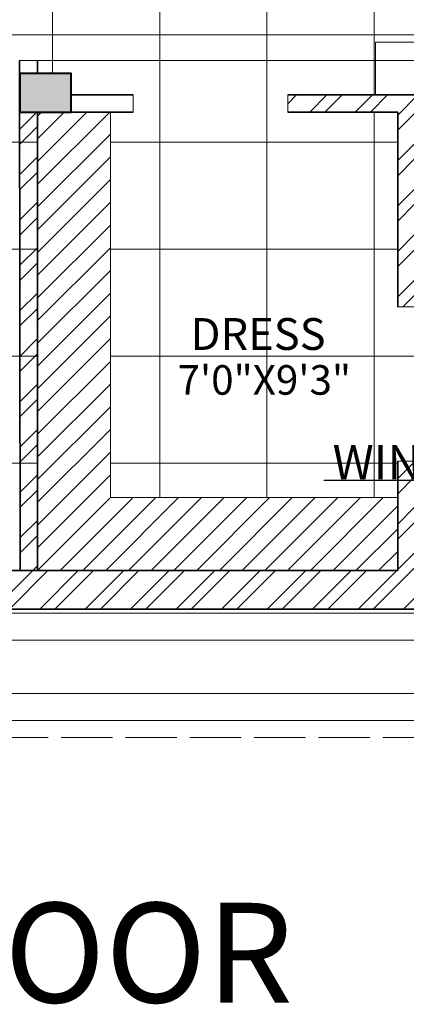
# Model space of a CAD drawing. Units: inches. Extents: x 351 to 1738, y -265 to 286.
# Tile 29 of 38: x 1380 to 1470, y -265 to -35. Entities that reach past the tile are written whole.
import ezdxf

# ---------------------------------------------------------------- set-up
doc = ezdxf.new("R2010")
doc.units = ezdxf.units.IN
doc.header["$MEASUREMENT"] = 0
doc.linetypes.add('ACAD_ISO02W100', pattern=[15, 12, -3])
for name, color, linetype, lineweight in [('A-ANNO-DIMS', 2, 'Continuous', 18), ('A-ANNO-TITL', 7, 'Continuous', 35), ('A-AREA-IDEN', 7, 'Continuous', 18), ('A-COLS', 7, 'Continuous', 40), ('A-COLS-PATT', 6, 'Continuous', 13), ('A-DOOR', 3, 'Continuous', 18), ('A-FLOR-CASE', 9, 'Continuous', 18), ('A-FLOR-CASE-PATT', 9, 'Continuous', 9), ('A-FLOR-OVHD', 1, 'ACAD_ISO02W100', 18), ('A-FLOR-PATT', 9, 'Continuous', 9), ('A-WALL', 7, 'Continuous', 35), ('A-WALL-PATT', 152, 'Continuous', 13)]:
    doc.layers.add(name, color=color, linetype=linetype, lineweight=lineweight)
doc.styles.add('Annotative', font='arial.ttf')
doc.styles.get("Standard").update_dxf_attribs({"font": 'arial.ttf'})
doc.dimstyles.get("Standard").update_dxf_attribs({"dimtxt": 8, "dimasz": 5, "dimexe": 0.18, "dimexo": 0.0625, "dimgap": 0.09, "dimtad": 1, "dimtoh": 1, "dimzin": 0, "dimdsep": 46, "dimlunit": 4, "dimtxsty": 'Standard', "dimcen": 0, "dimclre": 256, "dimadec": 0, "dimazin": 0, "dimtfac": 1, "dimtofl": 0, "dimtmove": 0, "dimatfit": 3, "dimfxl": 1, "dimtolj": 1, "dimtzin": 0, "dimlwe": -1, "dimarcsym": 0})

# ---------------------------------------------------------------- blocks, each defined once
blk = doc.blocks.new('CONSOLE-TV')
blk.add_lwpolyline([(0, 0), (61, 0), (61, 12.29), (0, 12.29)], close=True)
blk = doc.blocks.new('COL-9x12')
blk.add_lwpolyline([(0, 12), (0, 0), (9, 0), (9, 12)], close=True)
blk = doc.blocks.new('*D32')
at = {"layer": 'A-ANNO-DIMS', "transparency": 16777216}
for p, q in [((1557.64, -102), (1552.12, -102)), ((1557.64, -138), (1552.12, -138))]:
    blk.add_line(p, q, dxfattribs=at)
at = {"layer": 'A-ANNO-DIMS', "color": 0, "lineweight": -2, "transparency": 16777216}
for p, q in [((1552.3, -107), (1552.3, -133)), ((1552.3, -138), (1552.3, -143)), ((1552.3, -143), (1450.98, -143))]:
    blk.add_line(p, q, dxfattribs=at)
at = {"layer": 'A-ANNO-DIMS', "color": 0, "transparency": 16777216}
for points in [[(1551.47, -107), (1553.14, -107), (1552.3, -102)], [(1551.47, -133), (1553.14, -133), (1552.3, -138)]]:
    blk.add_solid(points, dxfattribs=at)
at = {"layer": 'Defpoints', "color": 0, "transparency": 16777216}
for p in [(1557.7, -102), (1552.3, -138), (1557.7, -138)]:
    blk.add_point(p, dxfattribs=at)
at = {"layer": 'A-ANNO-DIMS', "color": 0, "transparency": 16777216, "insert": (1501.6, -138.77), "char_height": 8, "attachment_point": 5}
blk.add_mtext('\\A1;WINDOW 3\'-0" TYP.', dxfattribs=at)
blk = doc.blocks.new('*D66')
at = {"layer": 'A-ANNO-DIMS', "transparency": 16777216}
for p, q in [((1384.27, -3.5), (1596.33, -3.5)), ((1384.27, -45), (1596.33, -45))]:
    blk.add_line(p, q, dxfattribs=at)
at = {"layer": 'A-ANNO-DIMS', "color": 0, "lineweight": -2, "transparency": 16777216}
blk.add_line((1596.15, -40), (1596.15, -8.5), dxfattribs=at)
at = {"layer": 'A-ANNO-DIMS', "color": 0, "transparency": 16777216}
for points in [[(1595.32, -8.5), (1596.99, -8.5), (1596.15, -3.5)], [(1595.32, -40), (1596.99, -40), (1596.15, -45)]]:
    blk.add_solid(points, dxfattribs=at)
at = {"layer": 'Defpoints', "color": 0, "transparency": 16777216}
for p in [(1384.2, -3.5), (1596.15, -3.5), (1384.2, -45)]:
    blk.add_point(p, dxfattribs=at)
at = {"layer": 'A-ANNO-DIMS', "color": 0, "transparency": 16777216, "insert": (1591.92, -24.25), "char_height": 8, "attachment_point": 5, "rotation": 90}
blk.add_mtext('\\A1;3\'-5 1/2"', dxfattribs=at)

msp = doc.modelspace()

# ---------------------------------------------------------------- hatches: boundary and pattern name
at = {"layer": 'A-COLS-PATT'}
h = msp.add_hatch(color=256, dxfattribs=at)
h.dxf.hatch_style = 1
h.paths.add_polyline_path([(1112.704, 237.963), (1103.704, 237.963), (1103.704, 228.963), (1112.704, 228.963)])
h.paths.add_polyline_path([(1115.704, 237.963), (1112.704, 237.963), (1112.704, 228.963), (1115.704, 228.963)])
h.paths.add_polyline_path([(1043.704, 255.963), (1034.704, 255.963), (1034.704, 243.963), (1043.704, 243.963)])
h.paths.add_polyline_path([(1043.704, 210.963), (1034.704, 210.963), (1034.704, 198.963), (1043.704, 198.963)])
h.paths.add_polyline_path([(1043.704, -45.037), (1034.704, -45.037), (1034.704, -57.037), (1043.704, -57.037)])
h.paths.add_polyline_path([(1112.704, -45.037), (1103.704, -45.037), (1103.704, -57.037), (1112.704, -57.037)])
h.paths.add_polyline_path([(1112.704, -161.037), (1103.704, -161.037), (1103.704, -164.037), (1103.704, -173.037), (1112.704, -173.037)])
h.paths.add_polyline_path([(1043.704, -161.037), (1034.704, -161.037), (1034.704, -173.037), (1043.704, -173.037)])
h.paths.add_polyline_path([(1248.549, -164.037), (1236.549, -164.037), (1236.549, -173.037), (1248.549, -173.037)])
h.paths.add_polyline_path([(1248.549, -50), (1236.549, -50), (1236.549, -59), (1248.549, -59)])
h.paths.add_polyline_path([(1248.704, 73.463), (1244.704, 73.463), (1244.704, 64.463), (1248.704, 64.463)])
h.paths.add_polyline_path([(1244.704, 73.463), (1236.704, 73.463), (1236.704, 64.463), (1244.704, 64.463)])
h.paths.add_polyline_path([(1248.704, 237.963), (1236.704, 237.963), (1236.704, 228.963), (1248.704, 228.963)])
h.paths.add_polyline_path([(1392.204, 237.963), (1380.204, 237.963), (1380.204, 228.963), (1392.204, 228.963)])
h.paths.add_polyline_path([(1536.064, 237.963), (1524.064, 237.963), (1524.064, 228.963), (1536.064, 228.963)])
h.paths.add_polyline_path([(1536.064, 73.463), (1524.064, 73.463), (1524.064, 64.463), (1536.064, 64.463)])
h.paths.add_polyline_path([(1384.204, 73.463), (1380.204, 73.463), (1380.204, 64.463), (1384.204, 64.463)])
h.paths.add_polyline_path([(1392.064, 73.463), (1384.204, 73.463), (1384.204, 64.463), (1392.064, 64.463)])
h.paths.add_polyline_path([(1536.064, -53.037), (1524.064, -53.037), (1524.064, -57.037), (1536.064, -57.037)])
h.paths.add_polyline_path([(1536.064, -48.037), (1524.064, -48.037), (1524.064, -53.037), (1536.064, -53.037)])
h.paths.add_polyline_path([(1392.064, -48.037), (1380.064, -48.037), (1380.064, -56.5), (1380.065, -57.037), (1392.064, -57.037)])
h.paths.add_polyline_path([(1536.064, -164.037), (1524.064, -164.037), (1524.064, -173.037), (1536.064, -173.037)])
at = {"layer": 'A-FLOR-CASE-PATT'}
h = msp.add_hatch(dxfattribs=at)
h.set_pattern_fill('ANSI31', color=256, scale=30)
h.set_pattern_definition([(45, (1384.204, -164.0373), (-2.65165, 2.65165), [])])
h.paths.add_polyline_path([(1401.204, -57.037), (1384.204, -57.037), (1384.204, -164.037), (1468.204, -164.037), (1468.204, -147.037), (1401.204, -147.037)])
at = {"layer": 'A-FLOR-PATT', "transparency": 33554559}
h = msp.add_hatch(dxfattribs=at)
h.set_pattern_fill('ANSI37', color=256, scale=200, angle=135)
h.set_pattern_definition([(180, (1112.704, -164.037), (-2e-15, -25), []), (270, (1112.704, -164.037), (25, -5e-15), [])])
h.paths.add_polyline_path([(1380.064, 73.463), (1380.132, 148.463), (1338.064, 148.463), (1290.704, 148.463), (1290.704, 88.463), (1248.704, 88.463), (1248.704, -2.009), (1244.704, -2.009), (1244.704, 142.457), (1160.704, 142.457), (1160.704, 158.963), (1160.704, 170.137), (1160.704, 206.137), (1160.704, 228.963), (1112.704, 228.963), (1112.704, 209.963), (1112.704, 168.963), (1124.704, 168.963), (1124.704, 162.963), (1112.704, 162.963), (1112.704, 64.463), (1112.704, 60.463), (1112.704, 0.463), (1112.704, -48.026), (1146.804, -47.981), (1146.804, -35.691), (1207.804, -35.691), (1207.804, -47.902), (1236.542, -47.864), (1236.544, -50.009), (1248.5, -50.009), (1248.506, -102.915), (1248.512, -150.915), (1248.514, -164.037), (1248.549, -164.037), (1273.017, -164.037), (1273.017, -128.799), (1355.24, -128.799), (1355.24, -164.037), (1384.204, -164.037), (1384.204, -57.037), (1380.064, -57.037), (1380.064, -48.037), (1392.064, -48.037), (1392.064, -53.037), (1406.549, -53.037), (1406.549, -57.037), (1401.204, -57.037), (1401.204, -147.037), (1468.204, -147.037), (1468.204, -138.5), (1472.204, -138.5), (1472.204, -102.5), (1468.204, -102.5), (1468.204, -57.037), (1442.549, -57.037), (1442.549, -53.037), (1463.049, -53.037), (1463.049, -40.747), (1524.049, -40.747), (1524.049, -48.037), (1536.064, -48.037), (1536.064, -53.037), (1557.704, -53.037), (1557.704, 204.963), (1384.204, 204.963), (1384.204, 73.463), (1392.064, 73.463), (1392.064, 64.463), (1384.204, 64.463), (1384.204, -3.5), (1380.204, -3.537), (1380.204, 64.463), (1380.064, 64.463)])
h.paths.add_polyline_path([(1510.714, 86.458, -0.1039845), (1511.661, 85.595, 0.4704384), (1510.158, 87.614, 0.0961001)], flags=16)
h.paths.add_polyline_path([(1510.443, 100.266, 0.009798), (1504.693, 100.48, 0.0287898), (1504.6, 99.767, -0.1653311), (1505.519, 96.135, -0.1436014)], flags=16)
h.paths.add_polyline_path([(1487.201, 85.595, -0.1039845), (1488.148, 86.458, 0.0961001), (1488.704, 87.614, 0.4704384)], flags=0)
h.paths.add_polyline_path([(1495.052, 100.43), (1494.178, 100.43, -0.0264629), (1494.262, 99.774, -0.1442193)], flags=16)
h.paths.add_polyline_path([(1444.485, 86.458, -0.1039845), (1445.433, 85.595, 0.4704384), (1443.93, 87.614, 0.0961001)], flags=16)
h.paths.add_polyline_path([(1420.972, 85.595, -0.1039845), (1421.92, 86.458, 0.0961001), (1422.475, 87.614, 0.4704384)], flags=16)
h.paths.add_polyline_path([(1428.632, 100.335, 0.0010541), (1427.971, 100.309, -0.0215241), (1428.033, 99.774, -0.1143008)], flags=16)
h.paths.add_polyline_path([(1419.906, 143.708, 0.0249793), (1420.222, 157.526), (1421.573, 159.101), (1421.573, 175.369), (1391.393, 175.369), (1391.393, 200.519), (1542.294, 200.519), (1542.294, 175.369), (1512.028, 175.369, 0.0198653), (1511.521, 153.838, 0.0251335), (1512.758, 118.323, 0.0205529), (1512.942, 115.253), (1419.834, 115.253, -0.0004142), (1419.843, 124.798), (1413.059, 124.798), (1413.059, 84.437, -0.0618528), (1415.831, 80.45, -0.0930773), (1420.972, 85.595, -0.2675367), (1422.371, 84.732, 0.0851103), (1424.052, 84.616, -0.8853927), (1424.033, 84.851, -1.1258145), (1424.073, 84.366, -0.0879871), (1422.371, 84.732, -0.2675367), (1422.326, 83.089, -0.3705421), (1420.972, 85.595, 0.0930773), (1415.831, 80.45, -0.0874142), (1417.914, 73.937), (1418.941, 73.937, 0.0272504), (1418.913, 76.906, -0.1157032), (1421.051, 73.937), (1445.354, 73.937, -0.1157032), (1447.492, 76.906, 0.0272504), (1447.464, 73.937), (1448.491, 73.937, -0.0874142), (1450.574, 80.45, 0.0930773), (1445.433, 85.595, -0.3705421), (1444.079, 83.089, -0.2675367), (1444.034, 84.732, -0.0879871), (1442.332, 84.366, -1.1258145), (1442.372, 84.851, -2.0327363), (1442.364, 84.368, 0.0863779), (1444.034, 84.732, -0.2675367), (1445.433, 85.595, -0.0930773), (1450.574, 80.45, -0.2577317), (1466.483, 90.927, -0.4786702), (1468.832, 91.907, -0.4786702), (1471.18, 90.927, -0.26264), (1483.053, 81.78, -0.0718662), (1487.201, 85.595, -0.2675367), (1488.6, 84.732, 0.0851103), (1490.28, 84.616, -0.8853927), (1490.262, 84.851, -1.1258145), (1490.301, 84.366, -0.0879871), (1488.6, 84.732, -0.2675367), (1488.554, 83.089, -0.3705421), (1487.201, 85.595, 0.0718662), (1483.053, 81.78, -0.1320648), (1484.143, 73.937), (1485.169, 73.937, 0.0272504), (1485.142, 76.906, -0.1157032), (1487.28, 73.937), (1511.582, 73.937, -0.1157032), (1513.72, 76.906, 0.0272504), (1513.693, 73.937), (1514.719, 73.937, -0.0874142), (1516.802, 80.45, 0.0930773), (1511.661, 85.595, -0.3705421), (1510.308, 83.089, -0.2675367), (1510.262, 84.732, -0.0879871), (1508.561, 84.366, -1.1258145), (1508.601, 84.851, -2.0327363), (1508.592, 84.368, 0.0863779), (1510.262, 84.732, -0.2675367), (1511.661, 85.595, -0.0930773), (1516.802, 80.45, -0.0618528), (1519.575, 84.437), (1519.575, 73.937), (1413.059, 73.937), (1413.059, 124.798), (1419.843, 124.798, -0.0008205)], flags=16)
h.paths.add_polyline_path([(1220.149, 54.133, -0.1039845), (1220.869, 53.476, 0.4704384), (1219.727, 55.011, 0.0961001)], flags=16)
h.paths.add_polyline_path([(1219.944, 64.626, 0.009798), (1215.574, 64.789, 0.0287898), (1215.503, 64.247, -0.1653311), (1216.201, 61.487, -0.1436014)], flags=16)
h.paths.add_polyline_path([(1209.779, 64.449, 0.0974459), (1209.339, 64.751), (1208.247, 64.751, 0.1273905), (1207.7, 64.326, 0.1715858), (1206.95, 61.475, -0.1588542), (1207.636, 59.45, 0.0158984), (1207.795, 59.218, 0.0615457), (1208.598, 59.616, 0.1754158), (1208.638, 60.099, -0.2847793), (1209.348, 62.472, 0.3262165)], flags=16)
h.paths.add_polyline_path([(1169.818, 54.133, -0.1039845), (1170.538, 53.476, 0.4704384), (1169.396, 55.011, 0.0961001)], flags=16)
h.paths.add_polyline_path([(1159.017, 62.472, 0.2847642), (1158.307, 60.099, -0.1754332), (1158.267, 59.616, 0.3929302), (1159.448, 64.449, -0.3262298)], flags=16)
h.paths.add_polyline_path([(1156.342, 58.239, -0.1783213), (1154.011, 55.31, -0.1747359), (1154.722, 55.233, -0.2008015), (1156.27, 56.086, 0.1269899), (1157.283, 58.991, -0.0912053)], flags=16)
h.paths.add_polyline_path([(1156.624, 61.413, 0.1572752), (1157.316, 64.247, 0.1696217)], flags=16)
h.paths.add_polyline_path([(1152.67, 54.133, -0.0961001), (1151.95, 53.476, 0.0640762), (1154.465, 54.384, 0.1990158)], flags=16)
h.paths.add_polyline_path([(1202.281, 53.476, -0.1039845), (1203, 54.133, 0.0961001), (1203.423, 55.011, 0.4704384)], flags=0)
h.paths.add_polyline_path([(1151.139, 97.64, 0.0249793), (1151.379, 108.141), (1152.406, 109.338), (1152.406, 121.701), (1129.47, 121.701), (1129.47, 140.814), (1244.149, 140.814), (1244.149, 121.701), (1221.148, 121.701, 0.0198653), (1220.763, 105.338, 0.0251335), (1221.703, 78.349, 0.0205529), (1221.843, 76.016), (1151.078, 76.016, -0.1287433), (1148.786, 65.037, 0.5393525), (1150.327, 64.171, -0.027594), (1163.481, 64.751, 0.0976954), (1163.04, 64.449, 0.3262165), (1163.471, 62.472, -0.2847765), (1164.181, 60.099, -0.1947567), (1165.846, 61.443, -0.1554021), (1165.172, 64.247, -0.1660224), (1165.869, 61.475, -0.1770142), (1167.852, 62.77, -0.4482027), (1169.974, 60.807, -0.3934987), (1167.679, 57.86, -0.8955483), (1168.438, 54.524, -0.3557668), (1166.218, 56.086, -0.066024), (1165.505, 57.539), (1165.251, 56.243, -0.3717324), (1164.02, 59.758, -0.3736141), (1163.04, 64.449, -0.0976954), (1163.481, 64.751, 0.0213538), (1153.294, 64.429, -0.1341826), (1156.695, 61.368, 0.1868727), (1154.636, 62.77, 0.4482027), (1152.514, 60.807, 0.4037263), (1154.905, 57.846, 0.7112192), (1153.334, 55, 0.5315397), (1151.95, 53.476, -0.2675367), (1153.013, 52.821, 0.0851103), (1154.29, 52.732, -0.8853927), (1154.276, 52.911, -1.1258145), (1154.306, 52.543, -0.0879871), (1153.013, 52.821, -0.2675367), (1152.978, 51.572, -0.3705421), (1151.95, 53.476, 0.0930773), (1148.043, 49.566, -0.0874142), (1149.626, 44.617), (1150.406, 44.617, 0.0272504), (1150.385, 46.873, -0.1157032), (1152.01, 44.617), (1170.478, 44.617, -0.1157032), (1172.103, 46.873, 0.0272504), (1172.082, 44.617), (1172.862, 44.617, -0.0874142), (1174.445, 49.566, 0.0930773), (1170.538, 53.476, -0.3705421), (1169.51, 51.572, -0.2675367), (1169.475, 52.821, -0.0879871), (1168.182, 52.543, -1.1258145), (1168.212, 52.911, -2.0327363), (1168.206, 52.544, 0.0863779), (1169.475, 52.821, -0.2675367), (1170.538, 53.476, -0.0930773), (1174.445, 49.566, -0.2577317), (1186.536, 57.528, -0.4786702), (1188.321, 58.273, -0.4786702), (1190.106, 57.528, -0.26264), (1199.128, 50.577, -0.0718662), (1202.281, 53.476, -0.2675367), (1203.344, 52.821, 0.0851103), (1204.621, 52.732, -0.8853927), (1204.607, 52.911, -1.1258145), (1204.637, 52.543, -0.0879871), (1203.344, 52.821, -0.2675367), (1203.309, 51.572, -0.3705421), (1202.281, 53.476, 0.0718662), (1199.128, 50.577, -0.1320648), (1199.957, 44.617), (1200.737, 44.617, 0.0272504), (1200.716, 46.873, -0.1157032), (1202.341, 44.617), (1220.809, 44.617, -0.1157032), (1222.434, 46.873, 0.0272504), (1222.413, 44.617), (1223.193, 44.617, -0.0874142), (1224.776, 49.566, 0.0930773), (1220.869, 53.476, -0.3705421), (1219.841, 51.572, -0.2675367), (1219.806, 52.821, -0.0879871), (1218.513, 52.543, -1.1258145), (1218.543, 52.911, -2.0327363), (1218.537, 52.544, 0.0863779), (1219.806, 52.821, -0.2675367), (1220.869, 53.476, -0.0930773), (1224.776, 49.566, -0.0618528), (1226.883, 52.597), (1226.883, 44.617), (1145.936, 44.617), (1145.936, 83.269), (1151.091, 83.269, -0.0008205)], flags=16)
h.paths.add_polyline_path([(1218.01, 57.86, -0.8955483), (1218.769, 54.524, -0.3557668), (1216.549, 56.086, -0.066024), (1215.836, 57.539), (1215.582, 56.243, -0.3717324), (1214.351, 59.758, -0.3736141), (1213.371, 64.449, 0.3262165), (1213.802, 62.472, -0.2847765), (1214.512, 60.099, -0.1947567), (1216.177, 61.443, -0.1799907), (1218.183, 62.77, -0.4482027), (1220.305, 60.807, -0.3934987)], flags=16)
h.paths.add_polyline_path([(1424.735, 91.363, -0.3934987), (1421.715, 95.241, -0.4482027), (1424.507, 97.824, -0.1799907), (1427.147, 96.077, -0.1947567), (1429.338, 94.309, -0.2847765), (1430.272, 97.432, 0.3262165), (1430.839, 100.034, -0.3736141), (1429.55, 93.861, -0.3717324), (1427.929, 89.235), (1427.596, 90.941, -0.066024), (1426.657, 89.029, -0.3557668), (1423.736, 86.973, -0.8955483)], flags=16)
h.paths.add_polyline_path([(1238.033, 131.257, -1), (1227.329, 131.257, -1)], flags=0)
h.paths.add_polyline_path([(1235.357, 131.257, -1), (1230.005, 131.257, -1)], flags=0)
h.paths.add_polyline_path([(1214.039, 54.243, 0.1543819), (1214.38, 53.992, 0.3589549), (1213.613, 54.016, 0.6039484), (1214.379, 53.657, 0.3713191), (1213.968, 52.872, 0.1879935), (1214.312, 52.809, -0.592455), (1213.953, 52.967, -0.2942791), (1214.083, 53.691, -1.3001871), (1213.881, 54.134, -0.2837621), (1214.469, 53.896, 1.1509396)], flags=16)
h.paths.add_polyline_path([(1212.091, 56.286, -0.4084338), (1211.337, 56.445, -0.0362594), (1211.098, 56.848, -0.2360976), (1211.59, 56.63, 0.0353445), (1211.835, 56.543, -0.4752408), (1212.091, 56.286, -0.4752408), (1212.438, 56.182, 0.0353445), (1212.631, 56.007, -0.2360976), (1213.056, 55.676, -0.0362594), (1212.588, 55.697, -0.4084338)], flags=16)
h.paths.add_polyline_path([(1211.469, 50.297, 0.296043), (1210.47, 50.527, 0.310883), (1211.931, 50.148, 0.0212546)], flags=16)
h.paths.add_polyline_path([(1213.739, 51.818, -0.0362594), (1213.271, 51.838, -0.4084337), (1212.774, 52.427, -0.0947856), (1212.293, 50.703, 1.1504738), (1212.911, 50.232, 0.1662877), (1213.265, 50.68, -0.0252543), (1212.603, 50.13, 1.0879317), (1212.471, 49.407, 0.1662877), (1213.02, 49.251, -0.016128), (1212.567, 49.563, -0.286859), (1212.217, 49.638, 0.0221563), (1212.046, 50.055, -0.6461302), (1212.185, 50.498, 0.0884116), (1212.732, 52.077, -1.1860374), (1213.121, 52.323, 0.0353445), (1213.314, 52.148, -0.2360976)], flags=16)
h.paths.add_polyline_path([(1212.094, 50.342, -0.0485241), (1211.54, 49.605, -1.1038339), (1211.397, 48.738, -0.7855147), (1211.683, 48.254, -0.3920429), (1210.948, 48.525, -0.3928194), (1210.561, 47.995, -0.592455), (1210.201, 48.153, -0.2942791), (1210.331, 48.877, -0.7041716), (1210.316, 49.592, -0.6793441), (1210.729, 50.112, 0.5636764)], flags=16)
h.paths.add_polyline_path([(1211.274, 49.829, -0.1398258), (1210.745, 49.859, -0.2178785), (1210.948, 49.509, -0.4985724)], flags=0)
h.paths.add_polyline_path([(1433.426, 81.49, -0.181571), (1434.245, 81.788, -0.0080665), (1433.726, 82.205, 0.0455784), (1432.755, 81.242, 0.1790113)], flags=16)
h.paths.add_polyline_path([(1434.146, 81.009, -0.1324418), (1433.645, 80.771, 0.2590893), (1433.234, 80.471, -0.1802109), (1433.392, 80.805, -0.1699398), (1432.758, 81.109, 0.0326525), (1433.273, 80.474, -0.4933627), (1434.046, 80.146, -0.3904966)], flags=16)
h.paths.add_polyline_path([(1434.83, 80.047, -0.9475376), (1435.294, 79.576, -0.2991282), (1434.625, 79.404, -0.2704392), (1435.01, 78.591, -0.592455), (1434.537, 78.382, -0.3928194), (1434.027, 79.08, -0.3920429), (1433.06, 78.723, -0.3520423), (1433.003, 79.197, -0.1972159), (1433.75, 79.734, -0.7136405), (1434.447, 79.939, -0.2147903), (1434.819, 80.475, 0.4088333), (1435.075, 80.803, -0.2261519)], flags=16)
h.paths.add_polyline_path([(1432.67, 81.217, -0.4542182), (1431.897, 79.923, -0.4144105), (1431.301, 80.035, 0.0161291), (1431.897, 80.445, 0.2795702), (1432.073, 80.871, -0.2895037), (1431.103, 81.321, -0.4144105), (1430.978, 81.915, 0.0161296), (1431.586, 81.521, 0.341293), (1432.125, 81.583, -0.8131856)], flags=16)
h.paths.add_polyline_path([(1429.893, 86.381, -0.9475376), (1430.358, 85.91, -0.1731062), (1429.984, 85.712, -0.0388172), (1431.625, 84.214, -0.0879005), (1432.097, 88.549, -0.0497684), (1431.254, 88.49, -0.2360976), (1431.814, 88.925, 0.0353445), (1432.067, 89.155, -0.4752408), (1432.524, 89.291, -0.4752408), (1432.86, 89.63, 0.0353445), (1433.182, 89.744, -0.2360976), (1433.83, 90.032, -0.0362594), (1433.516, 89.502, -0.4084338), (1432.524, 89.291, -0.3124239), (1432.106, 88.58, 0.0885594), (1431.625, 84.214, -0.4084337), (1430.971, 83.439, -0.0362594), (1430.355, 83.412, -0.2360976), (1430.914, 83.847, 0.0353445), (1431.168, 84.078, -0.4752408), (1431.625, 84.214, 0.0388172), (1429.984, 85.712, -0.3217316), (1429.333, 86.048, -0.32743), (1429.883, 86.809, 0.4088333), (1430.138, 87.138, -0.2261519)], flags=16)
h.paths.add_polyline_path([(1211.206, 58.616, -0.9997836), (1211.336, 59.323, -0.6149935)], flags=16)
h.paths.add_polyline_path([(1210.288, 49.429, 0.1543819), (1210.629, 49.178, 0.3589549), (1209.861, 49.202, 0.6039484), (1210.627, 48.843, -0.5348247), (1210.806, 49.295, 0.7483464)], flags=16)
h.paths.add_polyline_path([(1209.589, 51.828, -0.0087906), (1209.775, 51.753, 0.1122315), (1209.466, 52.019, 1.4188509), (1209.014, 51.708, -0.4587257), (1208.651, 51.073, -0.592455), (1208.291, 51.232, -0.2942791), (1208.421, 51.955, -1.3001871), (1208.219, 52.398, -0.2260052), (1208.719, 52.257, -0.4755189), (1209.158, 52.369, -1.4554994), (1209.603, 52.664, 0.4213049), (1209.191, 52.262, -0.5912116), (1208.979, 51.796, 0.4973986), (1209.773, 51.333, 0.6493116)], flags=16)
h.paths.add_polyline_path([(1208.029, 52.041, 0.5446671), (1208.832, 52.045, 0.220132)], flags=0)
h.paths.add_polyline_path([(1210.438, 51.425, -0.2041997), (1210.277, 52.018, 0.2708262), (1209.915, 52.897, 0.3241145)], flags=0)
h.paths.add_polyline_path([(1209.668, 52.407, -0.60139), (1208.99, 52.221, -0.3949159), (1208.248, 52.83, -0.8367916), (1208.651, 53.017, -0.3384876), (1209.039, 52.571, 0.1941379), (1209.191, 52.262, 0.4139945), (1209.712, 52.475, 0.5177103), (1210.503, 51.416, 0.401922), (1209.493, 50.93, 0.2063956), (1209.516, 50.165, -0.3194629), (1210.417, 51.418, -0.466635)], flags=16)
h.paths.add_polyline_path([(1206.601, 56.086, -0.3557668), (1204.381, 54.524, -0.9211983), (1205.236, 57.846, 0.2065693), (1207.614, 58.991, -0.1269899)], flags=16)
h.paths.add_polyline_path([(1435.487, 82.816, 0.5277653), (1436.615, 83.361, 0.5085402), (1437.05, 82.433, 0.592455), (1437.524, 82.641, 0.3312448), (1436.963, 83.548, 0.3878632), (1437.808, 83.626, 0.5929544), (1437.618, 84.176, 0.2260158), (1436.961, 83.99, 0.3182053), (1437.588, 84.854, 0.6893744), (1437.05, 84.991, 0.3357648), (1436.539, 84.41, -0.1569934), (1436.404, 84.065, -0.4346112), (1436.961, 83.99, -0.2147903), (1437.333, 84.526, 0.4088333), (1437.588, 84.854, -0.2261519), (1437.343, 84.097, -0.9475376), (1437.808, 83.626, -0.2991282), (1437.139, 83.455, -0.2704392), (1437.524, 82.641, -0.592455), (1437.05, 82.433, -0.3928194), (1436.541, 83.13, -0.4396601), (1435.475, 82.794, -0.174614), (1435.942, 82.244, -0.2063956), (1435.912, 81.237, -0.2708262), (1435.125, 82.208, 0.2079765), (1434.686, 82.904, -0.1964955)], flags=16)
h.paths.add_polyline_path([(1435.386, 84.832, 0.270811), (1434.91, 83.676, -0.2042174), (1434.699, 82.895, 0.3241145)], flags=0)
h.paths.add_polyline_path([(1435.68, 84.18, -0.2176564), (1435.554, 83.304, -0.1767045), (1436.236, 83.778, -0.3730364)], flags=0)
h.paths.add_polyline_path([(1435.566, 100.034, 0.3262165), (1436.133, 97.432, -0.2847765), (1437.067, 94.309, -0.1947567), (1439.258, 96.077, -0.1554021), (1438.371, 99.767, -0.1660224), (1439.289, 96.12, -0.1770142), (1441.897, 97.824, -0.4482027), (1444.69, 95.241, -0.3934987), (1441.67, 91.363, -0.8955483), (1442.669, 86.973, -0.3557668), (1439.748, 89.029, -0.066024), (1438.809, 90.941), (1438.476, 89.235, -0.3717324), (1436.855, 93.861, -0.3736141)], flags=16)
h.paths.add_polyline_path([(1191.252, 49.507, -0.2740221), (1190.658, 48.409, 0.2675367), (1191.311, 47.344, 0.3705421)], flags=0)
h.paths.add_polyline_path([(1190.301, 49.717, 0.1990158), (1188.619, 49.04, 0.0640762), (1191.252, 49.507, -0.0961001)], flags=0)
h.paths.add_polyline_path([(1189.518, 47.857, 1.1258145), (1189.676, 47.523, 2.0446052)], flags=0)
h.paths.add_polyline_path([(1464.974, 80.372, 0.2740221), (1465.756, 78.927, -0.0830131)], flags=0)
h.paths.add_polyline_path([(1464.974, 80.372, 0.3705421), (1464.897, 77.525, 0.5763244)], flags=0)
h.paths.add_polyline_path([(1464.974, 80.372, -0.4704384), (1467.284, 81.372, -0.0961001), (1466.226, 80.648, -0.1990158), (1468.439, 79.757, -0.0640762)], flags=0)
h.paths.add_polyline_path([(1189.511, 56.43, -0.2594668), (1188.321, 56.391, -0.2594668), (1187.13, 56.43, 0.0851103), (1188.193, 55.716, -0.8853927), (1188.27, 55.878, -1.1960133), (1188.355, 55.442, 0.1014587)], flags=0)
h.paths.add_polyline_path([(1188.321, 57.596, 0.0780722), (1187.678, 57.24, 0.0155503), (1188.321, 57.136, 0.0155503), (1188.964, 57.24, 0.0780722)], flags=0)
h.paths.add_polyline_path([(1190.164, 55.365, -0.5763244), (1190.106, 57.528, -0.1982945), (1188.321, 58.319, -0.1982945), (1186.536, 57.528, -0.5763244), (1186.477, 55.365, -0.3705421), (1186.536, 57.528, 0.1982945), (1188.321, 58.319, 0.1982945), (1190.106, 57.528, -0.3705421)], flags=0)
h.paths.add_polyline_path([(1188.372, 55.878, 1.1258145), (1188.529, 55.544, 2.0446052)], flags=0)
h.paths.add_polyline_path([(1186.341, 49.717, -0.0961001), (1185.389, 49.507, 0.0640762), (1188.022, 49.04, 0.1990158)], flags=0)
h.paths.add_polyline_path([(1185.389, 49.507, -0.2675367), (1185.984, 48.409, 0.0851103), (1187.046, 47.695, -0.8853927), (1187.123, 47.857, -1.1258145), (1186.966, 47.523, -0.0879871), (1185.984, 48.409, -0.2675367), (1185.331, 47.344, -0.3705421)], flags=0)
h.paths.add_polyline_path([(1399.441, 187.944, -1), (1413.525, 187.944, -1)], flags=0)
h.paths.add_polyline_path([(1402.962, 187.944, -1), (1410.004, 187.944, -1)], flags=0)
h.paths.add_polyline_path([(1357.663, -72.245), (1377.272, -72.245), (1377.272, -91.854), (1357.663, -91.854)], flags=16)
h.paths.add_polyline_path([(1467.256, 78.201, -1.1258145), (1467.049, 77.761, -2.0446052)], flags=0)
h.paths.add_polyline_path([(1468.822, 88.714, 0.9411249), (1469.106, 88.316, 1.1371523), (1468.765, 88.755, 0.890986), (1468.99, 88.245, 0.0948283), (1470.398, 89.481, -0.2675367), (1471.18, 90.927, -0.0281232), (1469.678, 90.547, -0.0287737), (1469.948, 90.311, -0.0203267), (1468.832, 90.41, -0.0203267), (1467.716, 90.311, -0.0287737), (1467.986, 90.547, -0.0281232), (1466.483, 90.927, -0.2675367), (1467.265, 89.481, 0.0851103), (1468.663, 88.542, -1.2023159)], flags=0)
h.paths.add_polyline_path([(1178.25, 124.523, -0.1199286), (1165.65, 124.145, -0.1073492), (1159.133, 124.446, -0.1028906), (1159.132, 130.465, -0.0748968), (1158.993, 137.956, 0.002027), (1167.844, 137.479, -0.07553), (1180.337, 137.666, -0.0758613), (1186.502, 137.688, -0.1409896), (1186.272, 130.046, -0.0954805), (1186.729, 124.748, -0.10603)], flags=0)
h.paths.add_polyline_path([(1469.225, 79.757, -0.1990158), (1471.437, 80.648, -0.0961001), (1470.379, 81.372, -0.4704384), (1472.689, 80.372, -0.3705421), (1472.766, 77.525, -0.2675367), (1471.907, 78.927, -0.0879863), (1470.615, 77.761, -1.1258491), (1470.408, 78.201, -2.0327363), (1470.642, 77.778, 0.0863779), (1471.907, 78.927, -0.2675367), (1472.689, 80.372, -0.0640762)], flags=0)
h.paths.add_polyline_path([(1430.423, 186.902, -0.0748968), (1430.24, 196.758, 0.002027), (1441.887, 196.131, -0.07553), (1458.326, 196.377, -0.0758613), (1466.438, 196.406, -0.1409896), (1466.136, 186.35, -0.0954805), (1466.737, 179.378, -0.10603), (1455.58, 179.082, -0.1199286), (1439, 178.585, -0.1073492), (1430.425, 178.981, -0.1028906)], flags=0)
h.paths.add_polyline_path([(1162.258, 49.939, 0.3357645), (1161.87, 49.497, -0.1569936), (1161.767, 49.235, -0.4346112), (1162.19, 49.178, -0.2147903), (1162.473, 49.585, 1.5291948)], flags=16)
h.paths.add_polyline_path([(1161.683, 49.021, 0.5815181), (1161.268, 49.583, 0.5927609)], flags=16)
h.paths.add_polyline_path([(1162.602, 48.058, 0.3713191), (1162.192, 48.843, 0.4345332), (1162.88, 48.962, 0.1850806), (1162.197, 48.926, 1.1218369)], flags=16)
h.paths.add_polyline_path([(1161.443, 48.941, -1.3071038), (1161.495, 48.571, -0.2177521), (1161.136, 48.254, 0.6973029), (1161.871, 49.048, 0.1215141)], flags=16)
h.paths.add_polyline_path([(1162.531, 49.429, -0.2070837), (1162.05, 49.146, -0.9920299)], flags=16)
h.paths.add_polyline_path([(1161.304, 49.578, -0.7196675), (1161.513, 50.079, -0.1304275), (1160.836, 50.168, 0.0395926)], flags=0)
h.paths.add_polyline_path([(1162.036, 50.584, -0.0080665), (1161.642, 50.9, 0.0293675), (1161.35, 50.297, -0.2057884)], flags=16)
h.paths.add_polyline_path([(1162.882, 51.392, -0.1247327), (1162.763, 51.828, -0.1011907), (1162.399, 51.438, -0.153425)], flags=0)
h.paths.add_polyline_path([(1164.235, 51.85, -0.3091075), (1164.513, 51.136, -0.6271245), (1163.781, 51.603, -0.6859091), (1162.777, 51.219, -0.2332851), (1163.303, 50.165, -0.2708262), (1162.705, 50.903, 0.2041997), (1162.381, 51.425, 0.204182), (1162.542, 52.018, -0.2708414), (1162.903, 52.897, -0.1272607), (1163.219, 52.529, -1.1686811), (1163.781, 52.587, -0.3291117), (1164.168, 53.017, -0.8367917), (1164.571, 52.83, -0.1933406), (1164.391, 52.338, -0.9475376), (1164.744, 51.981, -0.2991282)], flags=16)
h.paths.add_polyline_path([(1163.598, 51.937, -1.2629561), (1163.236, 51.831, 0.0125754), (1162.971, 51.721, 0.2306566), (1163.151, 52.407, -0.1648982), (1163.178, 52.661, -0.4493201), (1163.628, 52.262, -0.721477), (1164.154, 52.088, -0.8499982)], flags=0)
h.paths.add_polyline_path([(1161.613, 58.616, -0.9804131), (1161.525, 59.049, -2.9089348)], flags=16)
h.paths.add_polyline_path([(1160.252, 49.166, -0.4144105), (1159.799, 49.251, 0.0161291), (1160.252, 49.563, 0.2795702), (1160.386, 49.887, -0.2895037), (1159.649, 50.229, -0.4144105), (1159.554, 50.68, 0.0161296), (1160.015, 50.381, 0.6178854), (1160.526, 50.703, -0.0947856), (1160.045, 52.427, -0.1404436), (1159.682, 52.042, -0.0578559), (1159.3, 51.872, 0.5448433), (1160.046, 52.419, -0.0881216), (1160.404, 55.721, -0.0497684), (1159.763, 55.676, -0.2360976), (1160.188, 56.007, 0.0353445), (1160.381, 56.182, -0.4752408), (1160.728, 56.286, -0.4752408), (1160.984, 56.543, 0.0353445), (1161.229, 56.63, -0.2360976), (1161.721, 56.848, -0.0362594), (1161.482, 56.445, -0.4084338), (1160.728, 56.286, -0.3124239), (1160.411, 55.745, 0.0885594), (1160.045, 52.427, 0.1070813), (1160.634, 50.498, -0.4947977), (1160.839, 50.149, -0.4542182)], flags=16)
h.paths.add_polyline_path([(1160.666, 49.808, -2.0765276), (1160.828, 50.172, 0.0195861)], flags=0)
h.paths.add_polyline_path([(1158.439, 53.992, 0.1543819), (1158.78, 54.243, 0.7483463), (1158.262, 54.109, -0.3382251), (1158.492, 53.839, -0.1708158), (1159.124, 53.779, 0.4957286), (1158.938, 54.134, 0.2260157)], flags=16)
h.paths.add_polyline_path([(1160.045, 52.427, 0.0388172), (1158.798, 53.565, -0.1198178), (1158.574, 53.586, -0.3091075), (1158.851, 52.872, -0.1879935), (1158.506, 52.809, 0.592455), (1158.866, 52.967, 0.3312448), (1158.44, 53.657, 0.2012451), (1158.798, 53.565, -0.034023), (1159.901, 52.578, -0.0442527), (1159.698, 52.323, -0.4752408)], flags=16)
h.paths.add_polyline_path([(1336.926, -95.392), (1336.926, -117.945), (1291.82, -117.945), (1291.82, -95.392)], flags=16)
h.paths.add_polyline_path([(1357.535, -97.244), (1357.726, -96.697, 0.0348443)], flags=16)
h.paths.add_polyline_path([(1376.693, -96.478), (1377.301, -96.5, 0.0314968), (1375.907, -96.424), (1357.726, -96.424)], flags=16)
h.paths.add_polyline_path([(1379.403, -119.667, 0.0267056), (1380.043, -119.439, -0.0152991)], flags=16)
h.paths.add_polyline_path([(1357.726, -120.202), (1357.821, -120.202), (1357.821, -120.201)], flags=16)
h.paths.add_polyline_path([(1354.171, -104.592), (1354.469, -98.672, 0.0111377)], flags=16)
h.paths.add_polyline_path([(1355.058, -119.136), (1354.578, -118.539, 0.1431635)], flags=16)
h.paths.add_polyline_path([(1378.851, -96.821), (1378.85, -96.82), (1378.85, -96.82, -0.0496798), (1380.055, -97.191), (1378.85, -96.82, 0.1500541), (1375.135, -97.188), (1375.136, -119.44, -0.0099698), (1374.747, -116.649), (1357.726, -116.649, 0.1693849), (1357.535, -119.382), (1357.535, -119.382), (1357.535, -119.382, 0.0348176), (1357.726, -119.928), (1357.726, -119.928), (1357.726, -119.929, -0.0348772), (1357.535, -119.382), (1355.507, -119.382), (1355.317, -119.278), (1357.535, -119.382, -0.1693939), (1357.726, -116.649, -0.0391513), (1374.686, -116.113, -0.0020149), (1374.625, -115.546, 0.1153223), (1369.915, -115.474, 0.0609215), (1369.922, -101.154, 0.1151459), (1374.625, -101.079, -0.0020164), (1374.686, -100.513, -0.0391511), (1357.726, -99.977), (1374.747, -99.977, -0.0099633), (1375.135, -97.188), (1375.135, -97.188, -0.1501081)], flags=16)
h.paths.add_polyline_path([(1490.963, 91.363, -0.3934987), (1487.944, 95.241, -0.4482027), (1490.736, 97.824, -0.1799907), (1493.376, 96.077, -0.1947567), (1495.567, 94.309, -0.2847765), (1496.501, 97.432, 0.3262165), (1497.068, 100.034, -0.3736141), (1495.778, 93.861, -0.3717324), (1494.158, 89.235), (1493.824, 90.941, -0.066024), (1492.886, 89.029, -0.3557668), (1489.964, 86.973, -0.8955483)], flags=16)
h.paths.add_polyline_path([(1354.86, -97.658), (1355.316, -97.348, 0.1019112)], flags=16)
h.paths.add_polyline_path([(1497.063, 83.327, 0.1767244), (1496.37, 83.785, -0.4051388), (1496.016, 83.384, 0.4973986), (1497.06, 82.774, 0.6493116), (1496.818, 83.426, -0.0087906)], flags=16)
h.paths.add_polyline_path([(1496.339, 83.783, 0.5927609), (1496.886, 84.522, 0.5815181)], flags=16)
h.paths.add_polyline_path([(1495.11, 82.641, 0.592455), (1495.583, 82.433, 0.6769152), (1495.805, 83.59, 0.3756693)], flags=16)
h.paths.add_polyline_path([(1495.015, 84.176, -0.145057), (1495.301, 84.526, -0.4088333), (1495.045, 84.854, 0.2206292), (1495.381, 84.152, -0.199594), (1495.851, 83.764, -0.5240172), (1494.826, 83.626, -0.5929976)], flags=16)
h.paths.add_polyline_path([(1501.655, 81.915, -0.0161291), (1501.048, 81.521, -0.3927187), (1500.462, 81.37, -0.2106699), (1500.607, 81.142, 0.3066994)], flags=16)
h.paths.add_polyline_path([(1500.11, 89.291, -0.4084338), (1499.118, 89.502, -0.0362594), (1498.803, 90.032, -0.2360976), (1499.451, 89.744, 0.0353445), (1499.774, 89.63, -0.4752408), (1500.11, 89.291, -0.4752408), (1500.567, 89.155, 0.0353445), (1500.82, 88.925, -0.2360976), (1501.379, 88.49, -0.0362594), (1500.763, 88.516, -0.4084338)], flags=16)
h.paths.add_polyline_path([(1498.908, 82.205, -0.0513217), (1500.013, 81.134, -0.5879306), (1500.234, 81.676, 0.1070813), (1501.009, 84.214, -0.03529)], flags=16)
h.paths.add_polyline_path([(1496.93, 83.875, -0.2063956), (1497.247, 84.832, -0.2708262), (1497.724, 83.676, 0.2079765), (1497.944, 82.884, -0.3814554)], flags=16)
h.paths.add_polyline_path([(1496.721, 81.237, 0.2708125), (1497.509, 82.208, -0.2042157), (1497.935, 82.895, 0.3241145)], flags=16)
h.paths.add_polyline_path([(1497.529, 80.125, -0.145057), (1497.814, 80.475, -0.703182), (1498.282, 81.178, -0.1229248), (1497.977, 81.714, -0.2708368), (1499.207, 81.49, 0.2079641), (1499.993, 81.248, -0.2651454), (1499.278, 80.472, 0.3819006), (1498.808, 79.947, -0.3059049), (1498.848, 79.519, 0.4994816), (1498.574, 79.217, -0.4587257), (1498.097, 78.382, -0.592455), (1497.624, 78.591, -0.2704392), (1498.009, 79.404, -0.299116), (1497.34, 79.576, -0.5930157)], flags=16)
h.paths.add_polyline_path([(1500.736, 79.923, 0.4144105), (1501.333, 80.035, -0.3216484), (1500.192, 80.765, 0.0198856), (1499.976, 81.251, 0.4653307)], flags=16)
h.paths.add_polyline_path([(1501.009, 84.214, -0.0388172), (1502.649, 85.712, -0.1730946), (1502.276, 85.91, -0.5930157), (1502.465, 86.46, -0.145057), (1502.751, 86.809, -0.4088333), (1502.495, 87.138, 0.2206292), (1502.831, 86.436, -0.199594), (1503.301, 86.048, -0.3217316), (1502.649, 85.712, 0.0388172), (1501.009, 84.214, 0.1224486), (1501.412, 83.755, 0.4754908), (1501.335, 84.226, 0.055822), (1501.719, 83.847, -0.2360976), (1502.278, 83.412, -0.0362594), (1501.663, 83.439, -0.4084338)], flags=16)
h.paths.add_polyline_path([(1501.794, 100.034, 0.3262165), (1502.362, 97.432, -0.2847765), (1503.295, 94.309, -0.1947567), (1505.486, 96.077, -0.1799907), (1508.126, 97.824, -0.4482027), (1510.918, 95.241, -0.3934987), (1507.899, 91.363, -0.8955483), (1508.898, 86.973, -0.3557668), (1505.976, 89.029, -0.066024), (1505.038, 90.941), (1504.704, 89.235, -0.3717324), (1503.084, 93.861, -0.3736141)], flags=16)
h.paths.add_polyline_path([(1146.29, 131.257, -1), (1135.587, 131.257, -1)], flags=0)
h.paths.add_polyline_path([(1143.614, 131.257, -1), (1138.262, 131.257, -1)], flags=0)
h.paths.add_polyline_path([(1524.064, 73.463), (1536.064, 73.463), (1536.064, 64.463), (1524.064, 64.463)], flags=16)
h.paths.add_polyline_path([(1520.162, 187.944, -1), (1534.246, 187.944, -1)], flags=0)
h.paths.add_polyline_path([(1530.725, 187.944), (1527.204, 187.944), (1527.204, 184.423, 0.4142136)], flags=0)
h.paths.add_polyline_path([(1278.415, -91.154), (1331.067, -91.154), (1331.067, -80.583), (1278.415, -80.583)], flags=24)
h.paths.add_polyline_path([(1266.655, -79.354), (1354.738, -79.354), (1354.738, -67.817), (1266.655, -67.817)], flags=24)
h.paths.add_polyline_path([(1115.482, 206.184), (1155.098, 206.184), (1155.098, 217.714), (1115.482, 217.714)], flags=24)
h.paths.add_polyline_path([(1161.771, 8.501), (1222.466, 8.501), (1222.466, 19.079), (1161.771, 19.079)], flags=24)
h.paths.add_polyline_path([(1164.656, 18.795), (1210.615, 18.795), (1210.615, 30.324), (1164.656, 30.324)], flags=24)
h.paths.add_polyline_path([(1368.147, -32.882), (1379.362, -32.882), (1379.362, -21.733), (1368.147, -21.733)], flags=24)
h.paths.add_polyline_path([(1244.842, -31.012), (1256.057, -31.012), (1256.057, -19.863), (1244.842, -19.863)], flags=24)
h.paths.add_polyline_path([(1114.589, 195.739), (1156.517, 195.739), (1156.517, 206.31), (1114.589, 206.31)], flags=24)
h.paths.add_polyline_path([(1436.398, 37.632), (1505.131, 37.632), (1505.131, 48.203), (1436.398, 48.203)], flags=24)
h.paths.add_polyline_path([(1435.991, 47.919), (1507.906, 47.919), (1507.906, 59.456), (1435.991, 59.456)], flags=24)
h.paths.add_polyline_path([(1415.107, -124.896), (1457.038, -124.896), (1457.038, -114.318), (1415.107, -114.318)], flags=24)
h.paths.add_polyline_path([(1417.992, -114.602), (1457.609, -114.602), (1457.609, -103.073), (1417.992, -103.073)], flags=24)
h = msp.add_hatch(dxfattribs=at)
h.set_pattern_fill('ANSI32', color=256, scale=50, angle=135)
h.set_pattern_definition([(180, (1038.704, -199.037), (-2e-15, -18.75), []), (180, (1032.454, -192.787), (-2e-15, -18.75), [])])
h.paths.add_polyline_path([(1248.506, -102.915), (1236.559, -102.916), (1236.553, -56.864), (1112.704, -57.026), (1112.704, -57.037), (1103.704, -57.037), (1103.704, -45.037), (1103.704, 98.963), (1076.434, 98.963), (1076.549, -81.037), (1071.549, -81.037), (1043.704, -81.037), (1038.704, -81.037), (1038.704, -161.037), (1043.704, -161.037), (1043.704, -173.037), (1038.704, -173.037), (1038.704, -199.037), (1562.704, -199.037), (1562.704, -173.037), (1236.549, -173.037), (1236.549, -164.037), (1236.693, -164.037), (1236.676, -150.916), (1248.512, -150.915)])
h.paths.add_polyline_path([(1236.133, -134.078), (1247.348, -134.078), (1247.348, -122.929), (1236.133, -122.929)], flags=24)
h.paths.add_polyline_path([(1308.144, -185.548), (1321.66, -185.548), (1321.66, -174.4), (1308.144, -174.4)], flags=24)
h.paths.add_polyline_path([(1121.632, -122.88), (1179.647, -122.88), (1179.647, -112.309), (1121.632, -112.309)], flags=24)
h.paths.add_polyline_path([(1124.515, -112.593), (1177.986, -112.593), (1177.986, -101.056), (1124.515, -101.056)], flags=24)
h.paths.add_polyline_path([(1091.374, 23.58), (1104.89, 23.58), (1104.89, 34.728), (1091.374, 34.728)], flags=24)
at = {"layer": 'A-WALL-PATT'}
h = msp.add_hatch(dxfattribs=at)
h.set_pattern_fill('ANSI32', color=256, scale=20)
h.set_pattern_definition([(45, (1034.704, -173.037), (-5.3033, 5.3033), []), (45, (1038.24, -173.037), (-5.3033, 5.3033), [])])
h.paths.add_polyline_path([(1043.704, -57.037), (1034.704, -57.037), (1034.704, -81.037), (1043.704, -81.037)])
h.paths.add_polyline_path([(1043.704, 198.963), (1034.704, 198.963), (1034.704, -45.037), (1043.704, -45.037)])
h.paths.add_polyline_path([(1043.704, 243.963), (1034.704, 243.963), (1034.704, 237.963), (1034.704, 210.963), (1043.704, 210.963)])
h.paths.add_polyline_path([(1112.704, 255.963), (1043.704, 255.963), (1043.704, 246.963), (1103.704, 246.963), (1103.704, 237.963), (1112.704, 237.963), (1112.704, 251.963)])
h.paths.add_polyline_path([(1056.704, 207.963), (1043.704, 207.963), (1043.704, 198.963), (1056.704, 198.963)])
h.paths.add_polyline_path([(1103.704, 207.963), (1092.704, 207.963), (1092.704, 198.963), (1103.704, 198.963)])
h.paths.add_polyline_path([(1112.704, 228.963), (1103.704, 228.963), (1103.704, 74.963), (1112.704, 74.963), (1112.704, 97.5)])
h.paths.add_polyline_path([(1284.129, -164.037), (1248.549, -164.037), (1248.549, -173.037), (1284.129, -173.037)])
h.paths.add_polyline_path([(1524.064, -164.037), (1472.204, -164.037), (1472.204, -138.5), (1468.204, -138.5), (1468.204, -164.037), (1344.129, -164.037), (1344.129, -173.037), (1524.064, -173.037)])
h.paths.add_polyline_path([(1384.204, -57.037), (1380.065, -57.037), (1380.204, -164.037), (1384.204, -164.037)])
h.paths.add_polyline_path([(1566.704, -138), (1557.704, -138), (1557.704, -164.037), (1536.064, -164.037), (1536.064, -173.037), (1566.704, -173.037)])
h.paths.add_polyline_path([(1566.704, -30.189), (1557.704, -30.189), (1557.704, -53.037), (1536.064, -53.037), (1536.064, -57.037), (1557.704, -57.037), (1557.704, -102), (1566.704, -102)])
h.paths.add_polyline_path([(1524.064, -53.037), (1442.549, -53.037), (1442.549, -57.037), (1468.204, -57.037), (1468.204, -102.5), (1472.204, -102.5), (1472.204, -57.037), (1524.064, -57.037)])
h.paths.add_polyline_path([(1566.704, 120.993), (1557.704, 120.993), (1557.704, 29.811), (1566.704, 29.811)])
h.paths.add_polyline_path([(1384.204, 64.463), (1380.204, 64.463), (1380.204, -3.5), (1384.204, -3.5)])
h.paths.add_polyline_path([(1266.549, 237.963), (1248.704, 237.963), (1248.704, 228.963), (1266.549, 228.963)])
h.paths.add_polyline_path([(1329.549, 237.963), (1302.549, 237.963), (1302.549, 228.963), (1329.549, 228.963)])
h.paths.add_polyline_path([(1380.204, 237.963), (1365.549, 237.963), (1365.549, 228.963), (1380.204, 228.963)])
h.paths.add_polyline_path([(1524.064, 237.963), (1392.204, 237.963), (1392.204, 228.963), (1524.064, 228.963)])
h.paths.add_polyline_path([(1384.204, 228.963), (1380.204, 228.963), (1380.204, 73.463), (1384.204, 73.463)])
h.paths.add_polyline_path([(1566.704, 237.963), (1536.064, 237.963), (1536.064, 228.963), (1557.704, 228.963), (1557.704, 180.993), (1566.704, 180.993)])

# ---------------------------------------------------------------- linework, layer by layer
at = {"layer": 'A-DOOR'}
msp.add_line((1384.204, -45), (1380.049, -45), dxfattribs=at)
for points in [[(1406.549, -53.037), (1406.549, -57.037)], [(1442.549, -57.037), (1442.549, -53.037)], [(1472.204, -102.5), (1468.204, -102.5)], [(1468.204, -138.5), (1472.204, -138.5)]]:
    msp.add_lwpolyline(points, dxfattribs=at)
at = {"layer": 'A-FLOR-CASE'}
for p, q in [((1401.204, -57.037), (1401.204, -147.037)), ((1401.204, -147.037), (1468.204, -147.037))]:
    msp.add_line(p, q, dxfattribs=at)
at = {"layer": 'A-FLOR-OVHD'}
for p, q in [((1562.704, -199.037), (1038.704, -199.037)), ((1566.704, -203.037), (1034.704, -203.037))]:
    msp.add_line(p, q, dxfattribs=at)
at = {"layer": 'A-WALL'}
for p, q in [((1380.049, -45), (1380.204, -164.037)), ((1384.204, -45), (1384.204, -48.037)), ((1392.064, -53.037), (1406.549, -53.037)), ((1442.549, -53.037), (1524.064, -53.037)), ((1380.204, -57.037), (1406.549, -57.037)), ((1384.204, -57.037), (1384.204, -164.037)), ((1442.549, -57.037), (1468.204, -57.037)), ((1468.204, -57.037), (1468.204, -102.5)), ((1468.204, -138.5), (1468.204, -164.037)), ((1236.549, -164.037), (1468.204, -164.037)), ((1236.549, -173.037), (1566.704, -173.037))]:
    msp.add_line(p, q, dxfattribs=at)

# ---------------------------------------------------------------- block references
at = {"layer": 'A-COLS', "rotation": 90.00000000000006}
msp.add_blockref('COL-9x12', (1392.064, -57.038), dxfattribs=at)
at = {"layer": 'A-FLOR-CASE'}
msp.add_blockref('CONSOLE-TV', (1463.049, -53.037), dxfattribs=at)

# ---------------------------------------------------------------- texts
at = {"layer": 'A-ANNO-TITL', "style": 'Annotative'}
msp.add_text('DUPLEX THIRD FLOOR', height=23.27476, dxfattribs=at).set_placement((1115.071, -264.89))
at = {"layer": 'A-AREA-IDEN', "style": 'Annotative'}
for s, height, p in [('DRESS', 7.4326, (1419.914, -112.554)), ('7\'0"X9\'3"', 6.9014, (1416.87, -123.011))]:
    msp.add_text(s, height=height, dxfattribs=at).set_placement(p)

# ---------------------------------------------------------------- dimensions: what is measured, and where the dimension line sits
at = {"layer": 'A-ANNO-DIMS'}
dim = msp.add_linear_dim(base=(1596.154, -3.5), p1=(1384.204, -45), p2=(1384.204, -3.5), angle=90, dimstyle='Standard', override={"dimdec": 1, "dimlfac": 1, "dimrnd": 0, "dimzin": 1, "dimdsep": 46, "dimlunit": 4, "dimfrac": 2}, dxfattribs=at)
dim.commit()
dim.dimension.update_dxf_attribs({"geometry": '*D66', "text_midpoint": (1591.925, -24.25)})
dim = msp.add_linear_dim(base=(1552.304, -138), p1=(1557.704, -102), p2=(1557.704, -138), angle=270, text='WINDOW <> TYP.', dimstyle='Standard', override={"dimdec": 1, "dimlfac": 1, "dimrnd": 0, "dimzin": 1, "dimdsep": 46, "dimlunit": 4, "dimfrac": 2}, dxfattribs=at)
dim.commit()
dim.dimension.update_dxf_attribs({"geometry": '*D32', "text_midpoint": (1501.598, -138.768)})

doc.saveas('drawing.dxf')
